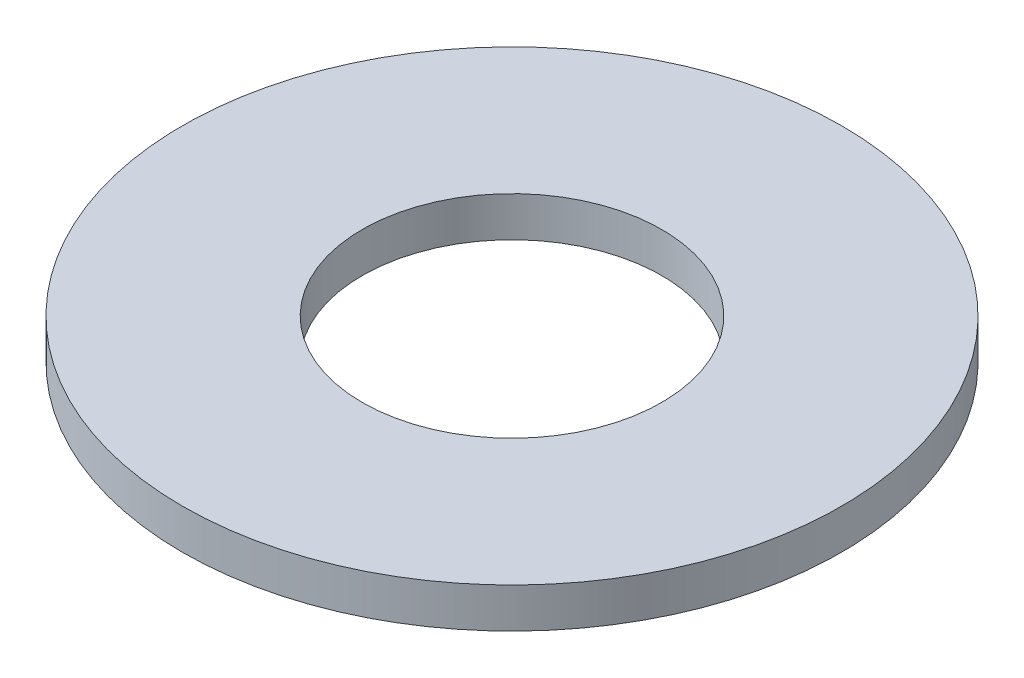
ISO-10303-21;
HEADER;
FILE_DESCRIPTION(('STEP AP214'),'2;1');
FILE_NAME('part.step','',(''),(''),'','','');
FILE_SCHEMA(('AUTOMOTIVE_DESIGN { 1 0 10303 214 1 1 1 1 }'));
ENDSEC;
DATA;
#1=APPLICATION_CONTEXT('core data for automotive mechanical design processes');
#2=APPLICATION_PROTOCOL_DEFINITION('international standard','automotive_design',2000,#1);
#3=PRODUCT_CONTEXT('',#1,'mechanical');
#4=PRODUCT('Part','Part','',(#3));
#5=PRODUCT_RELATED_PRODUCT_CATEGORY('part','',(#4));
#6=PRODUCT_DEFINITION_FORMATION('','',#4);
#7=PRODUCT_DEFINITION_CONTEXT('part definition',#1,'design');
#8=PRODUCT_DEFINITION('design','',#6,#7);
#9=PRODUCT_DEFINITION_SHAPE('','',#8);
#10=(LENGTH_UNIT() NAMED_UNIT(*) SI_UNIT(.MILLI.,.METRE.));
#11=(NAMED_UNIT(*) PLANE_ANGLE_UNIT() SI_UNIT($,.RADIAN.));
#12=(NAMED_UNIT(*) SI_UNIT($,.STERADIAN.) SOLID_ANGLE_UNIT());
#13=UNCERTAINTY_MEASURE_WITH_UNIT(LENGTH_MEASURE(1.E-05),#10,'distance_accuracy_value','');
#14=(GEOMETRIC_REPRESENTATION_CONTEXT(3) GLOBAL_UNCERTAINTY_ASSIGNED_CONTEXT((#13)) GLOBAL_UNIT_ASSIGNED_CONTEXT((#10,
#11,#12)) REPRESENTATION_CONTEXT('',''));
#15=CARTESIAN_POINT('',(0.,0.,0.));
#16=DIRECTION('',(0.,0.,1.));
#17=DIRECTION('',(1.,0.,0.));
#18=AXIS2_PLACEMENT_3D('',#15,#16,#17);
#19=CARTESIAN_POINT('',(0.,10.,0.));
#20=DIRECTION('',(0.,1.,0.));
#21=DIRECTION('',(0.,0.,1.));
#22=AXIS2_PLACEMENT_3D('',#19,#20,#21);
#23=PLANE('',#22);
#24=CARTESIAN_POINT('',(0.,10.,0.));
#25=DIRECTION('',(0.,1.,0.));
#26=DIRECTION('',(0.,0.,1.));
#27=AXIS2_PLACEMENT_3D('',#24,#25,#26);
#28=CIRCLE('',#27,82.5);
#29=CARTESIAN_POINT('',(0.,10.,82.5));
#30=VERTEX_POINT('',#29);
#31=EDGE_CURVE('E10',#30,#30,#28,.T.);
#32=ORIENTED_EDGE('',*,*,#31,.T.);
#33=EDGE_LOOP('',(#32));
#34=FACE_BOUND('',#33,.T.);
#35=CARTESIAN_POINT('',(0.,10.,0.));
#36=DIRECTION('',(0.,1.,0.));
#37=DIRECTION('',(0.,0.,1.));
#38=AXIS2_PLACEMENT_3D('',#35,#36,#37);
#39=CIRCLE('',#38,37.5);
#40=CARTESIAN_POINT('',(0.,10.,37.5));
#41=VERTEX_POINT('',#40);
#42=EDGE_CURVE('E48',#41,#41,#39,.T.);
#43=ORIENTED_EDGE('',*,*,#42,.F.);
#44=EDGE_LOOP('',(#43));
#45=FACE_BOUND('',#44,.T.);
#46=ADVANCED_FACE('F40',(#34,#45),#23,.T.);
#47=CARTESIAN_POINT('',(0.,0.,0.));
#48=DIRECTION('',(0.,1.,0.));
#49=DIRECTION('',(0.,0.,1.));
#50=AXIS2_PLACEMENT_3D('',#47,#48,#49);
#51=PLANE('',#50);
#52=CARTESIAN_POINT('',(0.,0.,0.));
#53=DIRECTION('',(0.,1.,0.));
#54=DIRECTION('',(0.,0.,1.));
#55=AXIS2_PLACEMENT_3D('',#52,#53,#54);
#56=CIRCLE('',#55,82.5);
#57=CARTESIAN_POINT('',(0.,0.,82.5));
#58=VERTEX_POINT('',#57);
#59=EDGE_CURVE('E41',#58,#58,#56,.T.);
#60=ORIENTED_EDGE('',*,*,#59,.F.);
#61=EDGE_LOOP('',(#60));
#62=FACE_BOUND('',#61,.T.);
#63=CARTESIAN_POINT('',(0.,0.,0.));
#64=DIRECTION('',(0.,1.,0.));
#65=DIRECTION('',(0.,0.,1.));
#66=AXIS2_PLACEMENT_3D('',#63,#64,#65);
#67=CIRCLE('',#66,37.5);
#68=CARTESIAN_POINT('',(0.,0.,37.5));
#69=VERTEX_POINT('',#68);
#70=EDGE_CURVE('E49',#69,#69,#67,.T.);
#71=ORIENTED_EDGE('',*,*,#70,.T.);
#72=EDGE_LOOP('',(#71));
#73=FACE_BOUND('',#72,.T.);
#74=ADVANCED_FACE('F58',(#62,#73),#51,.F.);
#75=CARTESIAN_POINT('',(0.,10.,0.));
#76=DIRECTION('',(0.,-1.,0.));
#77=DIRECTION('',(0.,0.,-1.));
#78=AXIS2_PLACEMENT_3D('',#75,#76,#77);
#79=CYLINDRICAL_SURFACE('',#78,82.5);
#80=ORIENTED_EDGE('',*,*,#31,.F.);
#81=EDGE_LOOP('',(#80));
#82=FACE_BOUND('',#81,.T.);
#83=ORIENTED_EDGE('',*,*,#59,.T.);
#84=EDGE_LOOP('',(#83));
#85=FACE_BOUND('',#84,.T.);
#86=ADVANCED_FACE('F39',(#82,#85),#79,.T.);
#87=CARTESIAN_POINT('',(0.,10.,0.));
#88=DIRECTION('',(0.,-1.,0.));
#89=DIRECTION('',(0.,0.,-1.));
#90=AXIS2_PLACEMENT_3D('',#87,#88,#89);
#91=CYLINDRICAL_SURFACE('',#90,37.5);
#92=ORIENTED_EDGE('',*,*,#42,.T.);
#93=EDGE_LOOP('',(#92));
#94=FACE_BOUND('',#93,.T.);
#95=ORIENTED_EDGE('',*,*,#70,.F.);
#96=EDGE_LOOP('',(#95));
#97=FACE_BOUND('',#96,.T.);
#98=ADVANCED_FACE('F57',(#94,#97),#91,.F.);
#99=CLOSED_SHELL('',(#46,#74,#86,#98));
#100=MANIFOLD_SOLID_BREP('B2',#99);
#101=ADVANCED_BREP_SHAPE_REPRESENTATION('',(#18,#100),#14);
#102=SHAPE_DEFINITION_REPRESENTATION(#9,#101);
ENDSEC;
END-ISO-10303-21;
